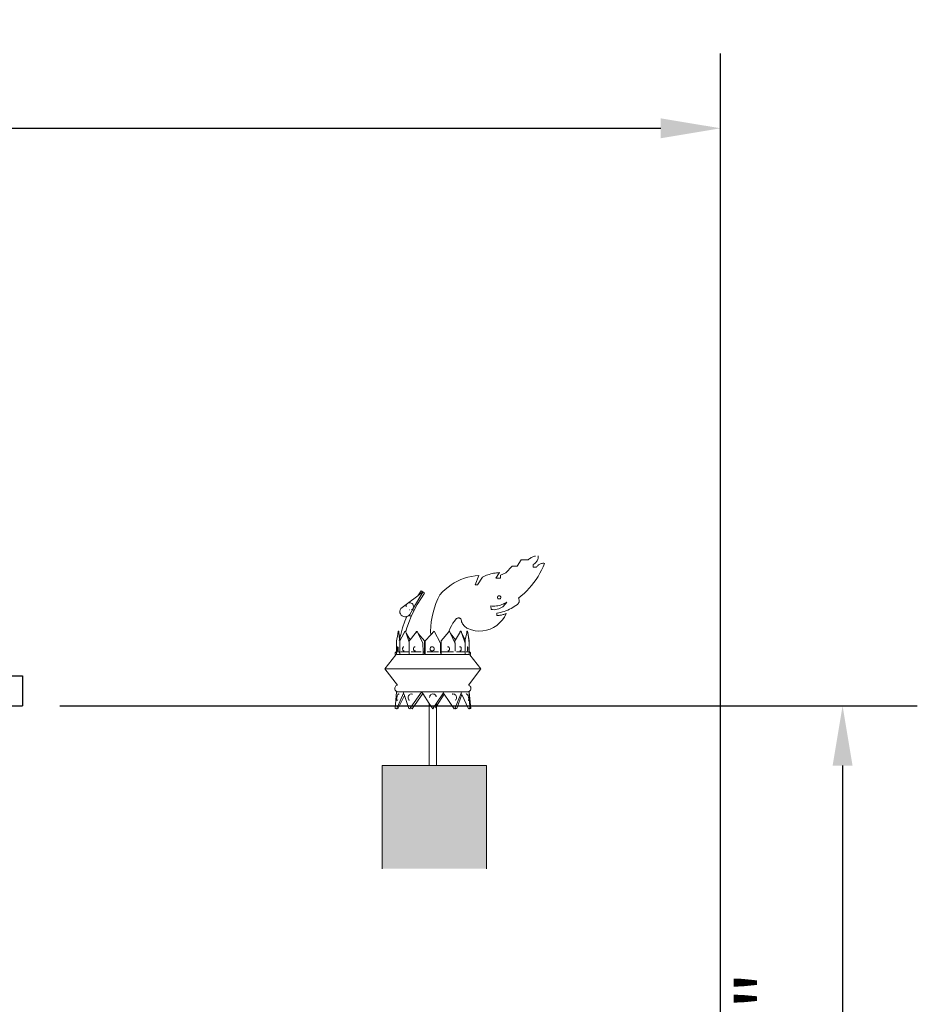
# Model space of a CAD drawing. Units: millimetres. Extents: x 7894 to 8038, y 6851 to 6951.
# Tile 48 of 49: x 7960.21 to 7975.23, y 6931.89 to 6948.36. Entities that reach past the tile are written whole.
import ezdxf

# ---------------------------------------------------------------- set-up
doc = ezdxf.new("R2010")
doc.units = ezdxf.units.MM
for name, color, linetype, lineweight in [('A-ANNO-DIMS', 2, 'Continuous', 18), ('A-FURN-ACCS', 8, 'Continuous', 13), ('A-FURN-SHLF', 7, 'Continuous', 30)]:
    doc.layers.add(name, color=color, linetype=linetype, lineweight=lineweight)
doc.layers.add('A-FURN-ACCS-PATT', color=116, linetype='Continuous', lineweight=9, true_color=0x136734)
doc.styles.get("Standard").update_dxf_attribs({"font": 'arial.ttf'})
doc.dimstyles.new('ISO-25', dxfattribs={"dimtxt": 1, "dimasz": 1, "dimexe": 1.25, "dimexo": 0.625, "dimtad": 1, "dimdec": 0, "dimlunit": 4, "dimtxsty": 'Standard', "dimcen": 2.5, "dimclrt": 1, "dimadec": 0, "dimazin": 0, "dimtfac": 1, "dimtdec": 0, "dimtmove": 0, "dimatfit": 3, "dimfxl": 1, "dimarcsym": 0})

# ---------------------------------------------------------------- blocks, each defined once
blk = doc.blocks.new('FLOATING-SHELF-ELEV')
for p, q in [((0, 0.5), (17.304, 0.5)), ((0, 0.5), (0, 0)), ((17.304, 0.5), (17.304, 0)), ((0, 0), (17.304, 0))]:
    blk.add_line(p, q)
blk = doc.blocks.new('DISPLAY-LEAF-FINIAL')
for p, q in [((2.409, 3.452), (2.421, 3.461)), ((2.421, 3.461), (2.434, 3.47)), ((2.434, 3.47), (2.447, 3.478)), ((2.447, 3.478), (2.461, 3.485)), ((2.461, 3.485), (2.475, 3.491)), ((2.475, 3.491), (2.489, 3.496)), ((2.489, 3.496), (2.504, 3.501)), ((2.504, 3.501), (2.519, 3.504)), ((2.56, 3.465), (2.556, 3.45)), ((2.563, 3.479), (2.56, 3.465)), ((2.565, 3.494), (2.563, 3.479)), ((2.565, 3.508), (2.565, 3.494)), ((2.023, 3.221), (2.127, 3.334)), ((2.127, 3.334), (2.209, 3.334)), ((2.209, 3.334), (2.276, 3.441)), ((2.276, 3.441), (2.398, 3.441)), ((2.398, 3.441), (2.409, 3.452)), ((2.493, 3.371), (2.48, 3.364)), ((2.48, 3.364), (2.48, 3.316)), ((2.48, 3.316), (2.533, 3.316)), ((2.505, 3.379), (2.493, 3.371)), ((2.516, 3.389), (2.505, 3.379)), ((2.527, 3.4), (2.516, 3.389)), ((2.536, 3.411), (2.527, 3.4)), ((2.533, 3.316), (2.54, 3.327)), ((2.544, 3.424), (2.536, 3.411)), ((2.54, 3.327), (2.549, 3.338)), ((2.551, 3.437), (2.544, 3.424)), ((2.549, 3.338), (2.558, 3.347)), ((2.556, 3.45), (2.551, 3.437)), ((2.558, 3.347), (2.569, 3.356)), ((2.569, 3.356), (2.58, 3.363)), ((2.58, 3.363), (2.592, 3.37)), ((2.592, 3.37), (2.604, 3.375)), ((2.604, 3.375), (2.617, 3.379)), ((2.617, 3.379), (2.63, 3.382)), ((2.646, 3.325), (2.62, 3.27)), ((2.63, 3.382), (2.643, 3.383)), ((2.643, 3.383), (2.657, 3.383)), ((2.67, 3.382), (2.646, 3.325)), ((2.657, 3.383), (2.67, 3.382)), ((1.27, 3.111), (1.328, 3.133)), ((1.328, 3.133), (1.388, 3.15)), ((1.388, 3.15), (1.449, 3.164)), ((1.449, 3.164), (1.51, 3.173)), ((1.51, 3.173), (1.572, 3.179)), ((1.572, 3.179), (1.511, 3.024)), ((1.55, 3.024), (1.632, 3.152)), ((1.632, 3.152), (1.654, 3.163)), ((1.654, 3.163), (1.676, 3.173)), ((1.676, 3.173), (1.699, 3.182)), ((1.699, 3.182), (1.722, 3.191)), ((1.722, 3.191), (1.745, 3.198)), ((1.745, 3.198), (1.769, 3.205)), ((1.769, 3.205), (1.793, 3.211)), ((1.793, 3.211), (1.817, 3.216)), ((1.817, 3.216), (1.841, 3.22)), ((1.841, 3.22), (1.865, 3.223)), ((1.914, 3.227), (1.854, 3.133)), ((1.854, 3.133), (1.934, 3.133)), ((1.865, 3.223), (1.889, 3.226)), ((1.889, 3.226), (1.914, 3.227)), ((1.934, 3.185), (2.023, 3.221)), ((1.934, 3.133), (1.934, 3.185)), ((2.56, 3.163), (2.527, 3.112)), ((2.591, 3.216), (2.56, 3.163)), ((2.62, 3.27), (2.591, 3.216)), ((1.007, 2.946), (1.055, 2.986)), ((1.055, 2.986), (1.105, 3.023)), ((1.105, 3.023), (1.158, 3.056)), ((1.158, 3.056), (1.213, 3.085)), ((1.213, 3.085), (1.27, 3.111)), ((1.511, 3.024), (1.55, 3.024)), ((2.413, 2.967), (2.371, 2.923)), ((2.453, 3.014), (2.413, 2.967)), ((2.491, 3.062), (2.453, 3.014)), ((2.527, 3.112), (2.491, 3.062)), ((0.547, 2.84), (0.379, 2.713)), ((0.634, 2.9), (0.463, 2.609)), ((0.605, 2.924), (0.547, 2.84)), ((0.634, 2.905), (0.547, 2.84)), ((0.599, 2.791), (0.663, 2.885)), ((0.634, 2.905), (0.605, 2.924)), ((0.634, 2.9), (0.634, 2.905)), ((0.663, 2.885), (0.634, 2.905)), ((0.92, 2.857), (0.884, 2.786)), ((0.92, 2.857), (0.962, 2.903)), ((0.962, 2.903), (1.007, 2.946)), ((1.883, 2.817), (1.885, 2.824)), ((1.883, 2.81), (1.883, 2.817)), ((1.885, 2.803), (1.883, 2.81)), ((1.885, 2.824), (1.889, 2.831)), ((1.888, 2.797), (1.885, 2.803)), ((1.889, 2.831), (1.894, 2.836)), ((1.894, 2.836), (1.9, 2.839)), ((1.9, 2.839), (1.907, 2.841)), ((1.907, 2.841), (1.914, 2.841)), ((1.914, 2.841), (1.921, 2.839)), ((1.921, 2.839), (1.928, 2.836)), ((1.928, 2.836), (1.933, 2.83)), ((1.933, 2.83), (1.937, 2.824)), ((1.936, 2.803), (1.933, 2.796)), ((1.938, 2.81), (1.936, 2.803)), ((1.937, 2.824), (1.938, 2.817)), ((1.938, 2.817), (1.938, 2.81)), ((2.281, 2.839), (2.233, 2.801)), ((2.327, 2.88), (2.281, 2.839)), ((2.371, 2.923), (2.327, 2.88)), ((0.379, 2.713), (0.264, 2.627)), ((0.353, 2.675), (0.358, 2.69)), ((0.353, 2.66), (0.353, 2.675)), ((0.353, 2.659), (0.353, 2.66)), ((0.353, 2.657), (0.353, 2.659)), ((0.358, 2.69), (0.367, 2.703)), ((0.367, 2.703), (0.379, 2.713)), ((0.379, 2.713), (0.393, 2.72)), ((0.393, 2.72), (0.409, 2.723)), ((0.409, 2.723), (0.425, 2.722)), ((0.425, 2.722), (0.44, 2.718)), ((0.44, 2.718), (0.453, 2.709)), ((0.453, 2.709), (0.464, 2.698)), ((0.464, 2.698), (0.471, 2.684)), ((0.471, 2.684), (0.475, 2.669)), ((0.474, 2.667), (0.475, 2.669)), ((0.474, 2.667), (0.475, 2.666)), ((0.541, 2.696), (0.488, 2.597)), ((0.541, 2.696), (0.599, 2.791)), ((0.826, 2.638), (0.804, 2.562)), ((0.853, 2.713), (0.826, 2.638)), ((0.884, 2.786), (0.853, 2.713)), ((1.793, 2.668), (1.77, 2.67)), ((1.77, 2.67), (1.776, 2.611)), ((1.816, 2.667), (1.793, 2.668)), ((1.84, 2.668), (1.816, 2.667)), ((1.863, 2.67), (1.84, 2.668)), ((1.886, 2.673), (1.863, 2.67)), ((1.909, 2.678), (1.886, 2.673)), ((1.894, 2.791), (1.888, 2.797)), ((1.9, 2.788), (1.894, 2.791)), ((1.907, 2.786), (1.9, 2.788)), ((1.914, 2.786), (1.907, 2.786)), ((1.931, 2.684), (1.909, 2.678)), ((1.921, 2.788), (1.914, 2.786)), ((1.928, 2.791), (1.921, 2.788)), ((1.949, 2.642), (1.926, 2.63)), ((1.933, 2.796), (1.928, 2.791)), ((1.954, 2.692), (1.931, 2.684)), ((1.97, 2.657), (1.949, 2.642)), ((1.975, 2.701), (1.954, 2.692)), ((1.99, 2.673), (1.97, 2.657)), ((1.996, 2.711), (1.975, 2.701)), ((2.007, 2.692), (1.99, 2.673)), ((2.017, 2.722), (1.996, 2.711)), ((2.023, 2.712), (2.007, 2.692)), ((2.036, 2.734), (2.017, 2.722)), ((2.036, 2.734), (2.023, 2.712)), ((2.137, 2.643), (2.11, 2.627)), ((2.164, 2.659), (2.137, 2.643)), ((2.19, 2.677), (2.164, 2.659)), ((2.216, 2.695), (2.19, 2.677)), ((2.223, 2.702), (2.216, 2.695)), ((2.23, 2.709), (2.223, 2.702)), ((2.235, 2.717), (2.23, 2.709)), ((2.233, 2.801), (2.238, 2.792)), ((2.24, 2.726), (2.235, 2.717)), ((2.238, 2.792), (2.242, 2.783)), ((2.243, 2.735), (2.24, 2.726)), ((2.242, 2.783), (2.245, 2.774)), ((2.245, 2.745), (2.243, 2.735)), ((2.245, 2.774), (2.246, 2.764)), ((2.246, 2.754), (2.245, 2.745)), ((2.246, 2.764), (2.246, 2.754)), ((0.253, 2.607), (0.249, 2.584)), ((0.249, 2.58), (0.249, 2.584)), ((0.249, 2.58), (0.251, 2.557)), ((0.251, 2.557), (0.259, 2.536)), ((0.264, 2.627), (0.253, 2.607)), ((0.259, 2.536), (0.272, 2.517)), ((0.272, 2.517), (0.29, 2.502)), ((0.29, 2.502), (0.311, 2.492)), ((0.311, 2.492), (0.334, 2.488)), ((0.363, 2.491), (0.332, 2.415)), ((0.334, 2.488), (0.358, 2.489)), ((0.358, 2.489), (0.363, 2.491)), ((0.363, 2.491), (0.38, 2.497)), ((0.365, 2.496), (0.363, 2.491)), ((0.38, 2.497), (0.4, 2.51)), ((0.398, 2.513), (0.402, 2.512)), ((0.398, 2.391), (0.44, 2.495)), ((0.403, 2.513), (0.4, 2.514)), ((0.4, 2.51), (0.402, 2.512)), ((0.402, 2.512), (0.403, 2.513)), ((0.402, 2.512), (0.44, 2.495)), ((0.403, 2.513), (0.415, 2.527)), ((0.403, 2.513), (0.44, 2.496)), ((0.409, 2.511), (0.408, 2.509)), ((0.42, 2.535), (0.409, 2.511)), ((0.414, 2.606), (0.413, 2.603)), ((0.461, 2.605), (0.415, 2.527)), ((0.44, 2.496), (0.486, 2.593)), ((0.443, 2.613), (0.446, 2.612)), ((0.451, 2.615), (0.449, 2.616)), ((0.463, 2.609), (0.461, 2.605)), ((0.486, 2.593), (0.461, 2.605)), ((0.463, 2.609), (0.488, 2.597)), ((0.787, 2.485), (0.774, 2.406)), ((0.804, 2.562), (0.787, 2.485)), ((1.801, 2.608), (1.776, 2.611)), ((1.827, 2.607), (1.801, 2.608)), ((1.852, 2.609), (1.827, 2.607)), ((1.878, 2.613), (1.852, 2.609)), ((1.903, 2.554), (1.872, 2.548)), ((1.872, 2.548), (1.872, 2.508)), ((1.872, 2.508), (1.885, 2.509)), ((1.902, 2.62), (1.878, 2.613)), ((1.885, 2.509), (1.898, 2.51)), ((1.898, 2.51), (1.911, 2.511)), ((1.926, 2.63), (1.902, 2.62)), ((1.934, 2.561), (1.903, 2.554)), ((1.911, 2.511), (1.924, 2.513)), ((1.924, 2.513), (1.937, 2.515)), ((1.964, 2.569), (1.934, 2.561)), ((1.937, 2.515), (1.95, 2.518)), ((1.95, 2.518), (1.963, 2.521)), ((1.997, 2.484), (1.961, 2.432)), ((1.963, 2.521), (1.976, 2.524)), ((1.994, 2.578), (1.964, 2.569)), ((1.976, 2.524), (1.988, 2.528)), ((1.988, 2.528), (2.001, 2.532)), ((2.024, 2.588), (1.994, 2.578)), ((2.026, 2.541), (1.997, 2.484)), ((2.001, 2.532), (2.013, 2.536)), ((2.013, 2.536), (2.026, 2.541)), ((2.053, 2.6), (2.024, 2.588)), ((2.082, 2.613), (2.053, 2.6)), ((2.11, 2.627), (2.082, 2.613)), ((0.332, 2.415), (0.295, 2.306)), ((0.361, 2.285), (0.398, 2.391)), ((0.766, 2.327), (0.763, 2.248)), ((0.774, 2.406), (0.766, 2.327)), ((1.113, 2.339), (1.092, 2.297)), ((1.136, 2.379), (1.113, 2.339)), ((1.163, 2.417), (1.136, 2.379)), ((1.193, 2.452), (1.163, 2.417)), ((1.198, 2.457), (1.193, 2.452)), ((1.204, 2.462), (1.198, 2.457)), ((1.211, 2.465), (1.204, 2.462)), ((1.218, 2.467), (1.211, 2.465)), ((1.225, 2.469), (1.218, 2.467)), ((1.232, 2.47), (1.225, 2.469)), ((1.239, 2.469), (1.232, 2.47)), ((1.247, 2.467), (1.239, 2.469)), ((1.254, 2.465), (1.247, 2.467)), ((1.26, 2.462), (1.254, 2.465)), ((1.266, 2.457), (1.26, 2.462)), ((1.271, 2.452), (1.266, 2.457)), ((1.274, 2.435), (1.271, 2.452)), ((1.278, 2.418), (1.274, 2.435)), ((1.283, 2.402), (1.278, 2.418)), ((1.29, 2.386), (1.283, 2.402)), ((1.298, 2.371), (1.29, 2.386)), ((1.308, 2.357), (1.298, 2.371)), ((1.319, 2.343), (1.308, 2.357)), ((1.331, 2.331), (1.319, 2.343)), ((1.343, 2.319), (1.331, 2.331)), ((1.357, 2.309), (1.343, 2.319)), ((1.372, 2.3), (1.357, 2.309)), ((1.816, 2.31), (1.759, 2.283)), ((1.87, 2.344), (1.816, 2.31)), ((1.918, 2.385), (1.87, 2.344)), ((1.961, 2.432), (1.918, 2.385)), ((0.213, 2.19), (0.195, 2.086)), ((0.213, 2.19), (0.215, 2.201)), ((0.215, 2.201), (0.22, 2.245)), ((0.223, 2.245), (0.215, 2.201)), ((0.223, 2.245), (0.22, 2.245)), ((0.223, 2.245), (0.23, 2.245)), ((0.232, 2.22), (0.23, 2.245)), ((0.232, 2.22), (0.25, 2.138)), ((0.244, 2.11), (0.232, 2.22)), ((0.317, 2.207), (0.248, 2.086)), ((0.263, 2.194), (0.25, 2.138)), ((0.295, 2.306), (0.263, 2.194)), ((0.297, 2.185), (0.292, 2.162)), ((0.317, 2.207), (0.33, 2.245)), ((0.338, 2.245), (0.317, 2.207)), ((0.332, 2.245), (0.33, 2.245)), ((0.344, 2.245), (0.338, 2.245)), ((0.347, 2.235), (0.344, 2.245)), ((0.347, 2.235), (0.361, 2.285)), ((0.354, 2.213), (0.347, 2.235)), ((0.354, 2.213), (0.42, 2.104)), ((0.404, 2.061), (0.354, 2.213)), ((0.507, 2.209), (0.42, 2.104)), ((0.507, 2.209), (0.525, 2.245)), ((0.532, 2.239), (0.507, 2.209)), ((0.528, 2.245), (0.525, 2.245)), ((0.528, 2.245), (0.532, 2.239)), ((0.537, 2.245), (0.532, 2.239)), ((0.54, 2.245), (0.537, 2.245)), ((0.556, 2.211), (0.54, 2.245)), ((0.548, 2.22), (0.556, 2.211)), ((0.556, 2.211), (0.663, 2.086)), ((0.636, 2.045), (0.556, 2.211)), ((0.765, 2.186), (0.671, 2.086)), ((0.763, 2.248), (0.765, 2.186)), ((0.821, 2.245), (0.765, 2.186)), ((0.93, 2.045), (0.821, 2.245)), ((1.07, 2.239), (0.939, 2.086)), ((1.07, 2.239), (1.069, 2.235)), ((1.071, 2.24), (1.07, 2.239)), ((1.07, 2.239), (1.071, 2.237)), ((1.075, 2.254), (1.071, 2.24)), ((1.074, 2.245), (1.071, 2.24)), ((1.074, 2.245), (1.078, 2.245)), ((1.092, 2.297), (1.075, 2.254)), ((1.095, 2.209), (1.078, 2.245)), ((1.095, 2.209), (1.182, 2.104)), ((1.095, 2.209), (1.171, 2.054)), ((1.248, 2.213), (1.182, 2.104)), ((1.248, 2.213), (1.258, 2.245)), ((1.265, 2.242), (1.248, 2.213)), ((1.258, 2.245), (1.264, 2.245)), ((1.264, 2.245), (1.265, 2.242)), ((1.267, 2.245), (1.265, 2.242)), ((1.267, 2.245), (1.272, 2.245)), ((1.285, 2.207), (1.272, 2.245)), ((1.285, 2.207), (1.344, 2.103)), ((1.285, 2.207), (1.34, 2.048)), ((1.37, 2.22), (1.344, 2.103)), ((1.37, 2.22), (1.372, 2.245)), ((1.375, 2.245), (1.37, 2.22)), ((1.387, 2.292), (1.372, 2.3)), ((1.372, 2.245), (1.375, 2.245)), ((1.375, 2.245), (1.382, 2.245)), ((1.382, 2.245), (1.389, 2.19)), ((1.447, 2.27), (1.387, 2.292)), ((1.389, 2.19), (1.408, 2.086)), ((1.407, 2.045), (1.389, 2.19)), ((1.509, 2.256), (1.447, 2.27)), ((1.572, 2.25), (1.509, 2.256)), ((1.635, 2.253), (1.572, 2.25)), ((1.698, 2.264), (1.635, 2.253)), ((1.759, 2.283), (1.698, 2.264)), ((0.195, 2.086), (0.195, 2.048)), ((0.195, 2.045), (0.195, 2.048)), ((0.195, 2.045), (0.195, 1.903)), ((0.208, 1.973), (0.209, 1.979)), ((0.209, 1.979), (0.211, 1.984)), ((0.211, 1.984), (0.213, 1.986)), ((0.212, 1.973), (0.213, 1.979)), ((0.216, 1.986), (0.213, 1.986)), ((0.213, 1.979), (0.214, 1.984)), ((0.214, 1.984), (0.216, 1.986)), ((0.219, 1.979), (0.218, 1.973)), ((0.22, 1.981), (0.219, 1.979)), ((0.22, 1.981), (0.219, 1.979)), ((0.244, 2.11), (0.239, 2.089)), ((0.25, 2.138), (0.244, 2.11)), ((0.248, 2.065), (0.244, 2.11)), ((0.248, 2.086), (0.248, 2.065)), ((0.248, 2.065), (0.248, 1.903)), ((0.25, 2.138), (0.256, 2.115)), ((0.3, 1.973), (0.304, 1.979)), ((0.304, 1.979), (0.308, 1.984)), ((0.308, 1.984), (0.314, 1.986)), ((0.316, 1.986), (0.314, 1.986)), ((0.42, 2.104), (0.404, 2.086)), ((0.404, 2.086), (0.404, 2.061)), ((0.404, 2.061), (0.404, 1.901)), ((0.482, 1.973), (0.488, 1.979)), ((0.488, 1.979), (0.495, 1.984)), ((0.495, 1.984), (0.502, 1.986)), ((0.504, 1.986), (0.502, 1.986)), ((0.636, 2.045), (0.637, 1.903)), ((0.663, 2.086), (0.663, 1.903)), ((0.671, 2.086), (0.671, 1.903)), ((0.761, 1.973), (0.767, 1.979)), ((0.767, 1.979), (0.775, 1.984)), ((0.775, 1.984), (0.784, 1.986)), ((0.784, 1.986), (0.793, 1.986)), ((0.793, 1.986), (0.802, 1.984)), ((0.802, 1.984), (0.81, 1.979)), ((0.81, 1.979), (0.816, 1.973)), ((0.93, 2.045), (0.931, 1.934)), ((0.939, 2.086), (0.939, 1.934)), ((1.044, 1.986), (1.046, 1.986)), ((1.046, 1.986), (1.054, 1.986)), ((1.054, 1.986), (1.062, 1.984)), ((1.062, 1.984), (1.069, 1.979)), ((1.069, 1.979), (1.075, 1.973)), ((1.182, 2.104), (1.171, 2.086)), ((1.171, 2.086), (1.171, 2.054)), ((1.176, 2.045), (1.171, 2.054)), ((1.176, 2.045), (1.177, 1.914)), ((1.249, 1.986), (1.251, 1.986)), ((1.251, 1.986), (1.257, 1.986)), ((1.257, 1.986), (1.263, 1.984)), ((1.263, 1.984), (1.268, 1.979)), ((1.268, 1.979), (1.272, 1.973)), ((1.344, 2.103), (1.34, 2.086)), ((1.34, 2.086), (1.34, 2.048)), ((1.341, 2.045), (1.34, 2.048)), ((1.341, 2.045), (1.342, 1.903)), ((1.373, 1.986), (1.376, 1.986)), ((1.376, 1.986), (1.378, 1.984)), ((1.376, 1.986), (1.377, 1.986)), ((1.377, 1.986), (1.379, 1.986)), ((1.378, 1.984), (1.379, 1.979)), ((1.379, 1.986), (1.381, 1.984)), ((1.379, 1.979), (1.381, 1.973)), ((1.381, 1.984), (1.383, 1.979)), ((1.383, 1.979), (1.384, 1.973)), ((1.408, 2.086), (1.407, 2.045)), ((1.407, 2.045), (1.408, 1.903)), ((0, 1.62), (0.181, 1.849)), ((0.17, 1.877), (0.172, 1.885)), ((0.17, 1.87), (0.17, 1.877)), ((0.172, 1.862), (0.17, 1.87)), ((0.172, 1.885), (0.176, 1.892)), ((0.175, 1.855), (0.172, 1.862)), ((0.181, 1.849), (0.175, 1.855)), ((0.176, 1.892), (0.182, 1.898)), ((0.182, 1.898), (0.189, 1.901)), ((0.189, 1.901), (0.195, 1.903)), ((0.195, 1.903), (0.195, 1.901)), ((0.195, 1.903), (0.196, 1.903)), ((0.195, 1.898), (0.195, 1.87)), ((0.195, 1.862), (0.195, 1.855)), ((0.195, 1.855), (0.195, 1.855)), ((0.205, 1.855), (0.195, 1.855)), ((0.196, 1.903), (0.198, 1.903)), ((0.196, 1.903), (0.197, 1.903)), ((0.237, 1.903), (0.198, 1.903)), ((0.205, 1.855), (0.205, 1.851)), ((0.248, 1.855), (0.205, 1.855)), ((0.205, 1.851), (0.205, 1.849)), ((0.207, 1.965), (0.208, 1.973)), ((0.207, 1.956), (0.207, 1.965)), ((0.207, 1.947), (0.207, 1.956)), ((0.207, 1.938), (0.207, 1.947)), ((0.208, 1.93), (0.207, 1.938)), ((0.209, 1.924), (0.208, 1.93)), ((0.211, 1.919), (0.209, 1.924)), ((0.21, 1.956), (0.211, 1.965)), ((0.21, 1.947), (0.21, 1.956)), ((0.211, 1.938), (0.21, 1.947)), ((0.211, 1.965), (0.212, 1.973)), ((0.212, 1.93), (0.211, 1.938)), ((0.213, 1.917), (0.211, 1.919)), ((0.213, 1.924), (0.212, 1.93)), ((0.216, 1.947), (0.213, 1.924)), ((0.214, 1.919), (0.213, 1.924)), ((0.214, 1.917), (0.213, 1.917)), ((0.216, 1.917), (0.214, 1.919)), ((0.216, 1.917), (0.214, 1.917)), ((0.217, 1.965), (0.216, 1.956)), ((0.216, 1.956), (0.216, 1.947)), ((0.216, 1.947), (0.217, 1.938)), ((0.218, 1.917), (0.216, 1.917)), ((0.218, 1.973), (0.217, 1.965)), ((0.218, 1.967), (0.217, 1.965)), ((0.217, 1.938), (0.218, 1.93)), ((0.218, 1.973), (0.218, 1.967)), ((0.218, 1.93), (0.219, 1.924)), ((0.219, 1.924), (0.22, 1.921)), ((0.221, 1.973), (0.22, 1.965)), ((0.22, 1.965), (0.22, 1.956)), ((0.22, 1.956), (0.22, 1.947)), ((0.22, 1.947), (0.22, 1.938)), ((0.22, 1.938), (0.221, 1.93)), ((0.222, 1.975), (0.221, 1.973)), ((0.221, 1.93), (0.222, 1.928)), ((0.24, 1.855), (0.24, 1.849)), ((0.248, 1.903), (0.244, 1.903)), ((0.245, 1.898), (0.244, 1.886)), ((0.248, 1.897), (0.244, 1.897)), ((0.248, 1.925), (0.246, 1.901)), ((0.248, 1.903), (0.248, 1.901)), ((0.248, 1.898), (0.248, 1.897)), ((0.248, 1.897), (0.248, 1.87)), ((0.248, 1.862), (0.248, 1.855)), ((0.248, 1.855), (0.276, 1.855)), ((0.391, 1.903), (0.265, 1.903)), ((0.275, 1.849), (0.276, 1.855)), ((0.276, 1.855), (0.405, 1.855)), ((0.295, 1.956), (0.297, 1.965)), ((0.295, 1.947), (0.295, 1.956)), ((0.297, 1.938), (0.295, 1.947)), ((0.297, 1.965), (0.3, 1.973)), ((0.3, 1.93), (0.297, 1.938)), ((0.303, 1.924), (0.3, 1.93)), ((0.308, 1.919), (0.303, 1.924)), ((0.313, 1.917), (0.308, 1.919)), ((0.319, 1.917), (0.313, 1.917)), ((0.322, 1.917), (0.319, 1.917)), ((0.404, 1.898), (0.404, 1.87)), ((0.404, 1.862), (0.405, 1.855)), ((0.405, 1.855), (0.637, 1.855)), ((0.439, 1.903), (0.607, 1.903)), ((0.476, 1.956), (0.478, 1.965)), ((0.476, 1.947), (0.476, 1.956)), ((0.478, 1.938), (0.476, 1.947)), ((0.478, 1.965), (0.482, 1.973)), ((0.482, 1.93), (0.478, 1.938)), ((0.488, 1.924), (0.482, 1.93)), ((0.495, 1.919), (0.488, 1.924)), ((0.502, 1.917), (0.495, 1.919)), ((0.51, 1.917), (0.502, 1.917)), ((0.512, 1.917), (0.51, 1.917)), ((0.637, 1.903), (0.634, 1.903)), ((0.637, 1.897), (0.634, 1.897)), ((0.637, 1.903), (0.637, 1.901)), ((0.663, 1.903), (0.637, 1.903)), ((0.637, 1.898), (0.637, 1.897)), ((0.637, 1.897), (0.637, 1.87)), ((0.663, 1.897), (0.637, 1.897)), ((0.637, 1.862), (0.637, 1.855)), ((0.663, 1.855), (0.637, 1.855)), ((0.663, 1.903), (0.671, 1.903)), ((0.663, 1.903), (0.663, 1.901)), ((0.663, 1.898), (0.663, 1.897)), ((0.663, 1.897), (0.663, 1.87)), ((0.671, 1.897), (0.663, 1.897)), ((0.663, 1.862), (0.663, 1.855)), ((0.671, 1.903), (0.671, 1.901)), ((0.671, 1.898), (0.671, 1.897)), ((0.671, 1.897), (0.671, 1.87)), ((0.671, 1.862), (0.671, 1.855)), ((0.671, 1.855), (0.932, 1.855)), ((0.708, 1.903), (0.894, 1.903)), ((0.754, 1.956), (0.756, 1.965)), ((0.754, 1.947), (0.754, 1.956)), ((0.756, 1.938), (0.754, 1.947)), ((0.756, 1.965), (0.761, 1.973)), ((0.761, 1.93), (0.756, 1.938)), ((0.767, 1.924), (0.761, 1.93)), ((0.775, 1.919), (0.767, 1.924)), ((0.784, 1.917), (0.775, 1.919)), ((0.793, 1.917), (0.784, 1.917)), ((0.802, 1.919), (0.793, 1.917)), ((0.81, 1.924), (0.802, 1.919)), ((0.816, 1.93), (0.81, 1.924)), ((0.816, 1.973), (0.821, 1.965)), ((0.821, 1.938), (0.816, 1.93)), ((0.821, 1.965), (0.823, 1.956)), ((0.823, 1.947), (0.821, 1.938)), ((0.823, 1.956), (0.823, 1.947)), ((0.939, 1.934), (0.931, 1.934)), ((0.931, 1.934), (0.931, 1.903)), ((0.931, 1.903), (0.931, 1.901)), ((0.939, 1.903), (0.931, 1.903)), ((0.931, 1.898), (0.931, 1.897)), ((0.931, 1.897), (0.932, 1.87)), ((0.939, 1.897), (0.931, 1.897)), ((0.932, 1.862), (0.932, 1.855)), ((0.939, 1.855), (0.932, 1.855)), ((0.942, 1.934), (0.939, 1.934)), ((0.939, 1.934), (0.939, 1.903)), ((0.942, 1.903), (0.939, 1.903)), ((0.939, 1.903), (0.939, 1.901)), ((0.939, 1.898), (0.939, 1.897)), ((0.942, 1.897), (0.939, 1.897)), ((0.939, 1.897), (0.939, 1.87)), ((0.939, 1.862), (0.939, 1.855)), ((1.342, 1.855), (0.939, 1.855)), ((0.953, 1.903), (1.146, 1.903)), ((1.022, 1.935), (1.021, 1.935)), ((1.052, 1.917), (1.054, 1.917)), ((1.062, 1.919), (1.054, 1.917)), ((1.069, 1.924), (1.062, 1.919)), ((1.075, 1.93), (1.069, 1.924)), ((1.075, 1.973), (1.079, 1.965)), ((1.079, 1.938), (1.075, 1.93)), ((1.079, 1.965), (1.081, 1.956)), ((1.081, 1.947), (1.079, 1.938)), ((1.081, 1.956), (1.081, 1.947)), ((1.33, 1.903), (1.197, 1.903)), ((1.254, 1.917), (1.257, 1.917)), ((1.263, 1.919), (1.257, 1.917)), ((1.268, 1.924), (1.263, 1.919)), ((1.272, 1.93), (1.268, 1.924)), ((1.272, 1.973), (1.275, 1.965)), ((1.275, 1.938), (1.272, 1.93)), ((1.275, 1.965), (1.276, 1.956)), ((1.276, 1.947), (1.275, 1.938)), ((1.276, 1.956), (1.276, 1.947)), ((1.347, 1.903), (1.342, 1.903)), ((1.342, 1.903), (1.342, 1.901)), ((1.342, 1.898), (1.342, 1.897)), ((1.347, 1.897), (1.342, 1.897)), ((1.342, 1.897), (1.342, 1.87)), ((1.342, 1.862), (1.342, 1.855)), ((1.408, 1.855), (1.342, 1.855)), ((1.356, 1.903), (1.4, 1.903)), ((1.378, 1.919), (1.375, 1.917)), ((1.375, 1.917), (1.379, 1.917)), ((1.379, 1.924), (1.378, 1.919)), ((1.381, 1.93), (1.379, 1.924)), ((1.381, 1.919), (1.379, 1.917)), ((1.381, 1.973), (1.382, 1.965)), ((1.382, 1.938), (1.381, 1.93)), ((1.383, 1.924), (1.381, 1.919)), ((1.382, 1.965), (1.382, 1.956)), ((1.382, 1.956), (1.382, 1.947)), ((1.382, 1.947), (1.382, 1.938)), ((1.384, 1.93), (1.383, 1.924)), ((1.384, 1.973), (1.385, 1.965)), ((1.385, 1.938), (1.384, 1.93)), ((1.385, 1.965), (1.386, 1.956)), ((1.386, 1.947), (1.385, 1.938)), ((1.386, 1.956), (1.386, 1.947)), ((1.408, 1.903), (1.413, 1.901)), ((1.408, 1.903), (1.408, 1.901)), ((1.408, 1.898), (1.408, 1.87)), ((1.408, 1.862), (1.408, 1.855)), ((1.413, 1.901), (1.42, 1.898)), ((1.42, 1.898), (1.426, 1.892)), ((1.427, 1.855), (1.421, 1.849)), ((1.421, 1.849), (1.602, 1.62)), ((1.426, 1.892), (1.43, 1.885)), ((1.431, 1.862), (1.427, 1.855)), ((1.43, 1.885), (1.432, 1.877)), ((1.433, 1.87), (1.431, 1.862)), ((1.432, 1.877), (1.433, 1.87)), ((0.207, 1.343), (0, 1.62)), ((1.602, 1.62), (0, 1.62)), ((1.602, 1.62), (1.395, 1.343)), ((0.168, 1.31), (0.174, 1.321)), ((0.174, 1.321), (0.183, 1.331)), ((0.183, 1.331), (0.195, 1.338)), ((0.195, 1.338), (0.207, 1.343)), ((1.395, 1.343), (1.408, 1.338)), ((1.408, 1.338), (1.419, 1.331)), ((1.419, 1.331), (1.428, 1.321)), ((1.428, 1.321), (1.434, 1.31)), ((0.164, 1.297), (0.168, 1.31)), ((0.164, 1.283), (0.164, 1.297)), ((0.167, 1.27), (0.164, 1.283)), ((0.173, 1.258), (0.167, 1.27)), ((0.171, 0.955), (0.191, 1.234)), ((0.182, 1.248), (0.173, 1.258)), ((0.193, 1.24), (0.182, 1.248)), ((0.219, 1.234), (0.191, 1.234)), ((0.206, 1.236), (0.193, 1.24)), ((0.196, 0.954), (0.311, 1.21)), ((0.202, 1.152), (0.206, 1.165)), ((0.219, 1.234), (0.206, 1.236)), ((0.206, 1.165), (0.212, 1.177)), ((0.212, 1.177), (0.217, 1.187)), ((0.215, 0.949), (0.324, 1.172)), ((0.217, 1.187), (0.223, 1.193)), ((0.219, 1.234), (0.297, 1.234)), ((0.223, 1.193), (0.228, 1.197)), ((0.228, 1.197), (0.232, 1.196)), ((0.232, 1.195), (0.232, 1.196)), ((0.232, 1.195), (0.237, 1.195)), ((0.297, 1.234), (0.302, 1.234)), ((0.303, 1.232), (0.297, 1.234)), ((0.303, 1.232), (0.302, 1.234)), ((0.302, 1.234), (0.594, 1.234)), ((0.311, 1.21), (0.303, 1.232)), ((0.324, 1.172), (0.311, 1.21)), ((0.402, 0.955), (0.324, 1.172)), ((0.389, 1.152), (0.395, 1.165)), ((0.395, 1.165), (0.403, 1.177)), ((0.403, 1.177), (0.413, 1.187)), ((0.413, 1.187), (0.424, 1.193)), ((0.424, 1.193), (0.436, 1.197)), ((0.434, 0.975), (0.609, 1.228)), ((0.436, 1.197), (0.448, 1.196)), ((0.448, 1.196), (0.458, 1.192)), ((0.455, 0.949), (0.632, 1.205)), ((0.458, 1.192), (0.461, 1.191)), ((0.594, 1.234), (0.617, 1.234)), ((0.609, 1.228), (0.594, 1.234)), ((0.617, 1.228), (0.617, 1.234)), ((0.952, 1.234), (0.617, 1.234)), ((0.632, 1.205), (0.617, 1.228)), ((0.742, 1.037), (0.632, 1.205)), ((0.748, 1.152), (0.752, 1.165)), ((0.752, 1.165), (0.76, 1.177)), ((0.76, 1.177), (0.77, 1.187)), ((0.77, 1.187), (0.783, 1.193)), ((0.783, 1.193), (0.797, 1.197)), ((0.797, 1.197), (0.812, 1.196)), ((0.812, 1.196), (0.826, 1.192)), ((0.826, 1.192), (0.838, 1.185)), ((0.838, 1.185), (0.848, 1.175)), ((0.848, 1.175), (0.855, 1.162)), ((0.855, 1.162), (0.859, 1.148)), ((0.86, 1.041), (0.977, 1.215)), ((0.86, 0.992), (0.99, 1.195)), ((0.981, 1.234), (0.952, 1.234)), ((0.977, 1.215), (0.974, 1.218)), ((0.99, 1.195), (0.977, 1.215)), ((0.981, 1.234), (0.982, 1.234)), ((0.982, 1.234), (0.983, 1.234)), ((1.284, 1.234), (0.983, 1.234)), ((1.16, 0.949), (0.99, 1.195)), ((1.124, 1.192), (1.126, 1.193)), ((1.126, 1.193), (1.127, 1.193)), ((1.127, 1.193), (1.138, 1.197)), ((1.138, 1.197), (1.15, 1.196)), ((1.15, 1.196), (1.162, 1.192)), ((1.162, 1.192), (1.174, 1.185)), ((1.174, 1.185), (1.184, 1.175)), ((1.177, 0.964), (1.275, 1.212)), ((1.184, 1.175), (1.191, 1.162)), ((1.191, 1.162), (1.196, 1.148)), ((1.202, 0.955), (1.285, 1.19)), ((1.275, 1.212), (1.283, 1.232)), ((1.285, 1.19), (1.275, 1.212)), ((1.283, 1.232), (1.29, 1.234)), ((1.283, 1.232), (1.284, 1.234)), ((1.284, 1.234), (1.29, 1.234)), ((1.398, 0.949), (1.285, 1.19)), ((1.29, 1.234), (1.383, 1.234)), ((1.359, 1.195), (1.364, 1.197)), ((1.359, 1.195), (1.362, 1.195)), ((1.364, 1.197), (1.369, 1.196)), ((1.369, 1.196), (1.374, 1.192)), ((1.374, 1.192), (1.38, 1.185)), ((1.38, 1.185), (1.386, 1.175)), ((1.397, 1.236), (1.383, 1.234)), ((1.41, 1.234), (1.383, 1.234)), ((1.386, 1.175), (1.392, 1.162)), ((1.392, 1.162), (1.396, 1.148)), ((1.409, 1.24), (1.397, 1.236)), ((1.42, 1.248), (1.409, 1.24)), ((1.411, 1.234), (1.41, 1.234)), ((1.411, 1.232), (1.411, 1.234)), ((1.435, 0.955), (1.411, 1.232)), ((1.42, 0.955), (1.411, 1.232)), ((1.429, 1.258), (1.42, 1.248)), ((1.435, 1.27), (1.429, 1.258)), ((1.434, 1.31), (1.438, 1.297)), ((1.438, 1.283), (1.435, 1.27)), ((1.438, 1.297), (1.438, 1.283)), ((0.194, 1.111), (0.196, 1.124)), ((0.195, 1.101), (0.194, 1.111)), ((0.196, 1.094), (0.195, 1.101)), ((0.196, 1.124), (0.198, 1.137)), ((0.199, 1.09), (0.196, 1.094)), ((0.198, 1.137), (0.202, 1.152)), ((0.203, 1.089), (0.199, 1.09)), ((0.204, 1.088), (0.203, 1.089)), ((0.211, 1.096), (0.213, 1.092)), ((0.213, 1.092), (0.214, 1.092)), ((0.214, 1.1), (0.214, 1.098)), ((0.387, 1.137), (0.389, 1.152)), ((0.387, 1.124), (0.387, 1.137)), ((0.391, 1.111), (0.387, 1.124)), ((0.397, 1.101), (0.391, 1.111)), ((0.406, 1.094), (0.397, 1.101)), ((0.409, 1.092), (0.406, 1.094)), ((0.742, 0), (0.742, 1.037)), ((0.799, 0.949), (0.742, 1.037)), ((0.747, 1.137), (0.748, 1.152)), ((0.747, 1.136), (0.747, 1.137)), ((0.816, 0.974), (0.86, 1.041)), ((0.843, 0.965), (0.86, 0.992)), ((0.859, 1.147), (0.859, 1.148)), ((0.86, 1.041), (0.86, 1.047)), ((0.86, 0.992), (0.86, 1.041)), ((0.86, 0), (0.86, 0.992)), ((1.174, 1.092), (1.172, 1.091)), ((1.174, 1.092), (1.175, 1.092)), ((1.185, 1.099), (1.175, 1.092)), ((1.192, 1.109), (1.185, 1.099)), ((1.196, 1.121), (1.192, 1.109)), ((1.196, 1.148), (1.198, 1.134)), ((1.198, 1.134), (1.196, 1.121)), ((1.392, 1.089), (1.39, 1.088)), ((1.39, 1.088), (1.395, 1.089)), ((1.399, 1.092), (1.395, 1.089)), ((1.396, 1.148), (1.4, 1.134)), ((1.401, 1.099), (1.399, 1.092)), ((1.4, 1.134), (1.402, 1.121)), ((1.402, 1.109), (1.401, 1.099)), ((1.402, 1.121), (1.402, 1.109)), ((0.194, 0.949), (0.171, 0.955)), ((0.194, 0.949), (0.196, 0.954)), ((0.215, 0.949), (0.196, 0.954)), ((0.416, 0.949), (0.402, 0.955)), ((0.416, 0.949), (0.434, 0.975)), ((0.442, 0.955), (0.434, 0.975)), ((0.455, 0.949), (0.442, 0.955)), ((0.799, 0.949), (0.816, 0.974)), ((0.816, 0.974), (0.814, 0.977)), ((0.816, 0.973), (0.816, 0.974)), ((1.16, 0.949), (1.173, 0.955)), ((1.173, 0.955), (1.177, 0.964)), ((1.187, 0.949), (1.177, 0.964)), ((1.187, 0.949), (1.202, 0.955)), ((1.398, 0.949), (1.41, 0.953)), ((1.41, 0.953), (1.42, 0.955)), ((1.412, 0.949), (1.41, 0.953)), ((1.412, 0.949), (1.435, 0.955))]:
    blk.add_line(p, q)
blk = doc.blocks.new('*D23')
at = {"layer": 'A-ANNO-DIMS', "color": 0, "lineweight": -2, "transparency": 16777216}
for p, q in [((7940.089, 6907.098), (7940.089, 6947.793)), ((7971.936, 6928.989), (7971.936, 6947.793)), ((7941.089, 6946.543), (7970.936, 6946.543))]:
    blk.add_line(p, q, dxfattribs=at)
at = {"layer": 'A-ANNO-DIMS', "color": 0, "transparency": 16777216}
for points in [[(7941.089, 6946.709), (7941.089, 6946.376), (7940.089, 6946.543)], [(7970.936, 6946.709), (7970.936, 6946.376), (7971.936, 6946.543)]]:
    blk.add_solid(points, dxfattribs=at)
at = {"layer": 'Defpoints', "color": 0, "transparency": 16777216}
for p in [(7971.936, 6946.543), (7971.936, 6928.364), (7940.089, 6906.473)]:
    blk.add_point(p, dxfattribs=at)
at = {"layer": 'A-ANNO-DIMS', "color": 1, "transparency": 16777216, "insert": (7956.012, 6947.678), "char_height": 1, "attachment_point": 5}
blk.add_mtext('2\'-8"', dxfattribs=at)
blk = doc.blocks.new('*D28')
at = {"layer": 'A-ANNO-DIMS', "color": 0, "lineweight": -2, "transparency": 16777216}
for p, q in [((7960.885, 6936.88), (7975.227, 6936.88)), ((7973.977, 6935.88), (7973.977, 6923.628)), ((7971.842, 6922.628), (7975.227, 6922.628))]:
    blk.add_line(p, q, dxfattribs=at)
at = {"layer": 'A-ANNO-DIMS', "color": 0, "transparency": 16777216}
for points in [[(7973.811, 6935.88), (7974.144, 6935.88), (7973.977, 6936.88)], [(7973.811, 6923.628), (7974.144, 6923.628), (7973.977, 6922.628)]]:
    blk.add_solid(points, dxfattribs=at)
at = {"layer": 'Defpoints', "color": 0, "transparency": 16777216}
for p in [(7960.26, 6936.88), (7971.217, 6922.628), (7973.977, 6922.628)]:
    blk.add_point(p, dxfattribs=at)
at = {"layer": 'A-ANNO-DIMS', "color": 1, "transparency": 16777216, "insert": (7972.835, 6929.754), "char_height": 1, "attachment_point": 5, "rotation": 90}
blk.add_mtext('1\'-2 1/2"', dxfattribs=at)

msp = doc.modelspace()

# ---------------------------------------------------------------- hatches: boundary and pattern name
at = {"layer": 'A-FURN-ACCS-PATT'}
h = msp.add_hatch(color=256, dxfattribs=at)
h.dxf.hatch_style = 1
h.paths.add_polyline_path([(7947.516, 6931.885), (7946.677, 6931.885), (7946.559, 6931.885), (7945.768, 6931.885), (7945.768, 6930.158), (7947.516, 6930.158)])
h.paths.add_polyline_path([(7947.485, 6922.447), (7946.646, 6922.447), (7946.528, 6922.447), (7945.737, 6922.447), (7945.737, 6920.72), (7947.485, 6920.72)])
h.paths.add_polyline_path([(7968.021, 6935.881), (7967.183, 6935.881), (7967.064, 6935.881), (7966.273, 6935.881), (7966.273, 6934.154), (7968.021, 6934.154)])
h.paths.add_polyline_path([(7960.61, 6924.856), (7959.771, 6924.856), (7959.652, 6924.856), (7958.862, 6924.856), (7958.862, 6923.128), (7960.61, 6923.128)])
h.paths.add_polyline_path([(7964.717, 6924.856), (7963.878, 6924.856), (7963.759, 6924.856), (7962.969, 6924.856), (7962.969, 6923.128), (7964.717, 6923.128)])
h.paths.add_polyline_path([(7971.07, 6924.856), (7970.231, 6924.856), (7970.112, 6924.856), (7969.322, 6924.856), (7969.322, 6923.128), (7971.07, 6923.128)])
h.paths.add_polyline_path([(7958.529, 6908.701), (7957.691, 6908.701), (7957.572, 6908.701), (7956.782, 6908.701), (7956.782, 6906.973), (7958.529, 6906.973)])

# ---------------------------------------------------------------- linework, layer by layer
at = {"layer": 'A-FURN-ACCS'}
for p, q in [((7966.273, 6934.154), (7966.273, 6935.881)), ((7966.273, 6935.881), (7967.064, 6935.881)), ((7967.183, 6935.881), (7967.064, 6935.881)), ((7967.183, 6935.881), (7968.021, 6935.881)), ((7968.021, 6934.154), (7968.021, 6935.881))]:
    msp.add_line(p, q, dxfattribs=at)

# ---------------------------------------------------------------- block references
msp.add_blockref('DISPLAY-LEAF-FINIAL', (7966.322, 6935.881), dxfattribs=at)
at = {"layer": 'A-FURN-SHLF'}
msp.add_blockref('FLOATING-SHELF-ELEV', (7942.957, 6936.88), dxfattribs=at)

# ---------------------------------------------------------------- dimensions: what is measured, and where the dimension line sits
at = {"layer": 'A-ANNO-DIMS'}
dim = msp.add_linear_dim(base=(7971.936, 6946.543), p1=(7940.089, 6906.473), p2=(7971.936, 6928.364), dimstyle='ISO-25', override={"dimdec": 1, "dimlfac": 1, "dimrnd": 0, "dimzin": 1, "dimdsep": 46, "dimlunit": 4, "dimfrac": 2}, dxfattribs=at)
dim.commit()
dim.dimension.update_dxf_attribs({"geometry": '*D23', "text_midpoint": (7956.012, 6947.678)})
dim = msp.add_linear_dim(base=(7973.977, 6922.628), p1=(7960.26, 6936.88), p2=(7971.217, 6922.628), angle=90, dimstyle='ISO-25', override={"dimdec": 1, "dimlfac": 1, "dimrnd": 0, "dimzin": 1, "dimdsep": 46, "dimlunit": 4, "dimfrac": 2}, dxfattribs=at)
dim.commit()
dim.dimension.update_dxf_attribs({"geometry": '*D28', "text_midpoint": (7972.835, 6929.754)})

doc.saveas('drawing.dxf')
